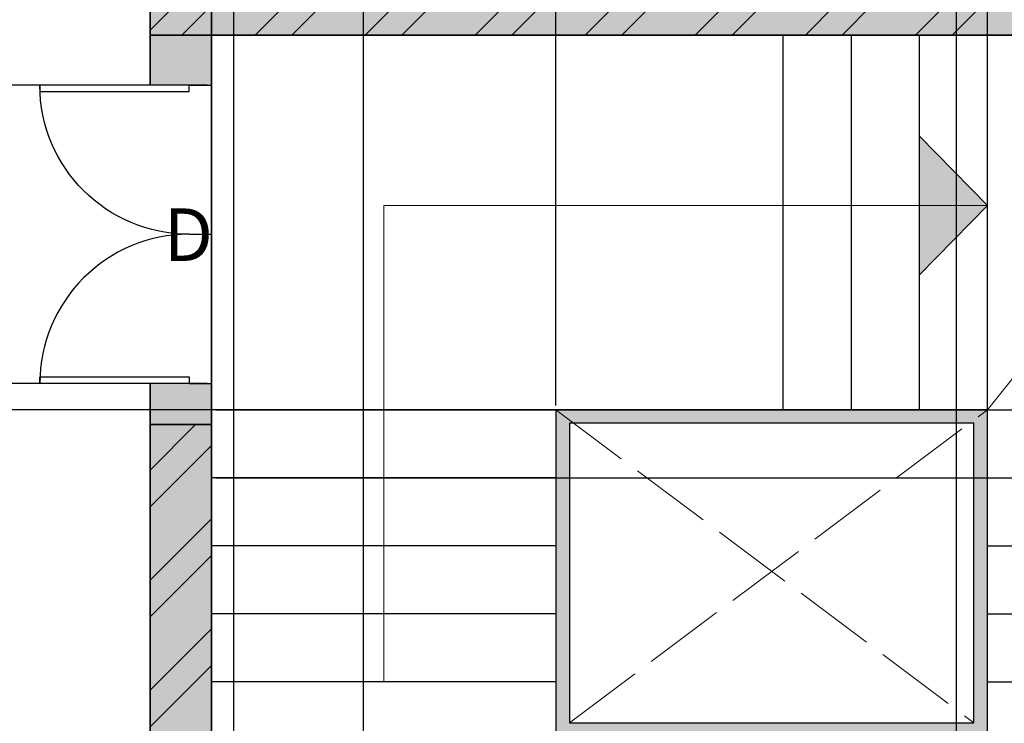
# Model space of a CAD drawing. Units: inches. Extents: x 1804 to 3296, y 909 to 2477.
# Tile 8 of 31: x 2130 to 2275, y 1226 to 1329. Entities that reach past the tile are written whole.
import ezdxf

# ---------------------------------------------------------------- set-up
doc = ezdxf.new("R2010")
doc.units = ezdxf.units.IN
doc.linetypes.add('ACAD_ISO02W100', pattern=[15, 12, -3])
for name, color, linetype, lineweight in [('A-ANNO-DIMS', 2, 'Continuous', 18), ('A-ANNO-SYMB', 7, 'Continuous', 18), ('A-ANNO-TTLB', 156, 'Continuous', 35), ('A-FLOR-PATT', 8, 'Continuous', 13), ('A-FLOR-STRS', 7, 'Continuous', 25), ('A-FLOR-STRS-OVHD', 8, 'ACAD_ISO02W100', 18), ('A-WALL-PATT', 10, 'Continuous', 13), ('DOOR', 30, 'Continuous', 25), ('TEXT', 190, 'Continuous', 18), ('WALL', 10, 'Continuous', 35)]:
    doc.layers.add(name, color=color, linetype=linetype, lineweight=lineweight)
doc.styles.get("Standard").update_dxf_attribs({"font": 'arial.ttf'})
doc.dimstyles.new('ISO-25', dxfattribs={"dimtxt": 5, "dimasz": 2.5, "dimexe": 1.25, "dimexo": 0.625, "dimtad": 1, "dimdec": 0, "dimlunit": 4, "dimtxsty": 'Standard', "dimcen": 2.5, "dimadec": 0, "dimazin": 0, "dimtfac": 1, "dimtdec": 0, "dimtmove": 0, "dimatfit": 3, "dimfxl": 1, "dimarcsym": 0})
pattern_1 = [(45, (0, 196.207), (-8.08223, 8.08223), []), (45, (5.388, 196.207), (-8.08223, 8.08223), [])]

# ---------------------------------------------------------------- blocks, each defined once
blk = doc.blocks.new('*U2')
for p, q in [((0, 0), (0, -6)), ((40, 0), (40, -6))]:
    blk.add_line(p, q)
blk.add_lwpolyline([(0, 0), (0, 40), (1.75, 40), (1.75, 0)], close=True)
blk.add_arc((0, 0), 40, 0, 90)
blk = doc.blocks.new('*D56')
at = {"layer": 'A-ANNO-DIMS', "color": 0, "lineweight": -2, "transparency": 16777216}
for p, q in [((2180.87, 1680.42), (2180.87, 975.89)), ((2268, 1680.42), (2268, 975.89)), ((2183.37, 977.14), (2265.5, 977.14))]:
    blk.add_line(p, q, dxfattribs=at)
at = {"layer": 'A-ANNO-DIMS', "color": 0, "lineweight": 100, "transparency": 16777216}
for points in [[(2183.37, 977.56), (2183.37, 976.72), (2180.87, 977.14)], [(2265.5, 977.56), (2265.5, 976.72), (2268, 977.14)]]:
    blk.add_solid(points, dxfattribs=at)
at = {"layer": 'Defpoints', "color": 0, "lineweight": 100, "transparency": 16777216}
for p in [(2180.87, 1681.04), (2268, 1681.04), (2268, 977.14)]:
    blk.add_point(p, dxfattribs=at)
at = {"layer": 'A-ANNO-DIMS', "color": 0, "transparency": 16777216, "insert": (2224.44, 980.32), "char_height": 5, "attachment_point": 5}
blk.add_mtext('7\'-3"', dxfattribs=at)
blk = doc.blocks.new('*D59')
at = {"layer": 'A-ANNO-DIMS', "color": 0, "lineweight": -2, "transparency": 16777216}
for p, q in [((2121.83, 1590.3), (2121.83, 975.89)), ((2161.83, 1590.3), (2161.83, 975.89)), ((2124.33, 977.14), (2159.33, 977.14))]:
    blk.add_line(p, q, dxfattribs=at)
at = {"layer": 'A-ANNO-DIMS', "color": 0, "lineweight": 100, "transparency": 16777216}
for points in [[(2124.33, 977.56), (2124.33, 976.72), (2121.83, 977.14)], [(2159.33, 977.56), (2159.33, 976.72), (2161.83, 977.14)]]:
    blk.add_solid(points, dxfattribs=at)
at = {"layer": 'Defpoints', "color": 0, "lineweight": 100, "transparency": 16777216}
for p in [(2121.83, 1590.92), (2161.83, 1590.92), (2161.83, 977.14)]:
    blk.add_point(p, dxfattribs=at)
at = {"layer": 'A-ANNO-DIMS', "color": 0, "transparency": 16777216, "insert": (2141.83, 980.32), "char_height": 5, "attachment_point": 5}
blk.add_mtext('3\'-4"', dxfattribs=at)
blk = doc.blocks.new('*D63')
at = {"layer": 'A-ANNO-DIMS', "color": 0, "lineweight": -2, "transparency": 16777216}
for p, q in [((2157.95, 1319.33), (1880.63, 1319.33)), ((1881.88, 1277.99), (1881.88, 1316.83)), ((2157.95, 1275.49), (1880.63, 1275.49))]:
    blk.add_line(p, q, dxfattribs=at)
at = {"layer": 'A-ANNO-DIMS', "color": 0, "lineweight": 100, "transparency": 16777216}
for points in [[(1881.47, 1316.83), (1882.3, 1316.83), (1881.88, 1319.33)], [(1881.47, 1277.99), (1882.3, 1277.99), (1881.88, 1275.49)]]:
    blk.add_solid(points, dxfattribs=at)
at = {"layer": 'Defpoints', "color": 0, "lineweight": 100, "transparency": 16777216}
for p in [(1881.88, 1319.33), (2158.58, 1319.33), (2158.58, 1275.49)]:
    blk.add_point(p, dxfattribs=at)
at = {"layer": 'A-ANNO-DIMS', "color": 0, "transparency": 16777216, "insert": (1878.7, 1297.41), "char_height": 5, "attachment_point": 5, "rotation": 90}
blk.add_mtext('3\'-8"', dxfattribs=at)
blk = doc.blocks.new('*D70')
at = {"layer": 'A-ANNO-DIMS', "color": 0, "lineweight": -2, "transparency": 16777216}
for p, q in [((2208.56, 1271.63), (1880.63, 1271.63)), ((1881.88, 1226.13), (1881.88, 1269.13)), ((2208.56, 1223.63), (1880.63, 1223.63))]:
    blk.add_line(p, q, dxfattribs=at)
at = {"layer": 'A-ANNO-DIMS', "color": 0, "lineweight": 100, "transparency": 16777216}
for points in [[(1881.47, 1269.13), (1882.3, 1269.13), (1881.88, 1271.63)], [(1881.47, 1226.13), (1882.3, 1226.13), (1881.88, 1223.63)]]:
    blk.add_solid(points, dxfattribs=at)
at = {"layer": 'Defpoints', "color": 0, "lineweight": 100, "transparency": 16777216}
for p in [(1881.88, 1271.63), (2209.19, 1271.63), (2209.19, 1223.63)]:
    blk.add_point(p, dxfattribs=at)
at = {"layer": 'A-ANNO-DIMS', "color": 0, "transparency": 16777216, "insert": (1878.7, 1247.63), "char_height": 5, "attachment_point": 5, "rotation": 90}
blk.add_mtext('4\'-0"', dxfattribs=at)
blk = doc.blocks.new('*D71')
at = {"layer": 'A-ANNO-DIMS', "color": 0, "lineweight": -2, "transparency": 16777216}
for p, q in [((2158.58, 1272.26), (2158.58, 1874.99)), ((2209.19, 1272.26), (2209.19, 1874.99)), ((2161.08, 1873.74), (2206.69, 1873.74))]:
    blk.add_line(p, q, dxfattribs=at)
at = {"layer": 'A-ANNO-DIMS', "color": 0, "lineweight": 100, "transparency": 16777216}
for points in [[(2161.08, 1874.15), (2161.08, 1873.32), (2158.58, 1873.74)], [(2206.69, 1874.15), (2206.69, 1873.32), (2209.19, 1873.74)]]:
    blk.add_solid(points, dxfattribs=at)
at = {"layer": 'Defpoints', "color": 0, "lineweight": 100, "transparency": 16777216}
for p in [(2209.19, 1873.74), (2158.58, 1271.63), (2209.19, 1271.63)]:
    blk.add_point(p, dxfattribs=at)
at = {"layer": 'A-ANNO-DIMS', "color": 0, "transparency": 16777216, "insert": (2183.88, 1876.95), "char_height": 5, "attachment_point": 5}
blk.add_mtext('4\'-2 1/2"', dxfattribs=at)
blk = doc.blocks.new('*D72')
at = {"layer": 'A-ANNO-DIMS', "color": 0, "lineweight": -2, "transparency": 16777216}
for p, q in [((2369.24, 1271.63), (2369.24, 1292.56)), ((2159.2, 1271.63), (2370.49, 1271.63)), ((2369.24, 1264.13), (2369.24, 1269.13)), ((2159.2, 1261.63), (2370.49, 1261.63))]:
    blk.add_line(p, q, dxfattribs=at)
at = {"layer": 'A-ANNO-DIMS', "color": 0, "lineweight": 100, "transparency": 16777216}
for points in [[(2368.82, 1269.13), (2369.65, 1269.13), (2369.24, 1271.63)], [(2368.82, 1264.13), (2369.65, 1264.13), (2369.24, 1261.63)]]:
    blk.add_solid(points, dxfattribs=at)
at = {"layer": 'Defpoints', "color": 0, "lineweight": 100, "transparency": 16777216}
for p in [(2158.58, 1271.63), (2369.24, 1271.63), (2158.58, 1261.63)]:
    blk.add_point(p, dxfattribs=at)
at = {"layer": 'A-ANNO-DIMS', "color": 0, "transparency": 16777216, "insert": (2366.06, 1283.35), "char_height": 5, "attachment_point": 5, "rotation": 90}
blk.add_mtext('0\'-10"', dxfattribs=at)
blk = doc.blocks.new('*D73')
at = {"layer": 'A-ANNO-DIMS', "color": 0, "lineweight": -2, "transparency": 16777216}
for p, q in [((2272.59, 1272.26), (2272.59, 1874.99)), ((2316.54, 1272.26), (2316.54, 1874.99)), ((2275.09, 1873.74), (2314.04, 1873.74))]:
    blk.add_line(p, q, dxfattribs=at)
at = {"layer": 'A-ANNO-DIMS', "color": 0, "lineweight": 100, "transparency": 16777216}
for points in [[(2275.09, 1874.15), (2275.09, 1873.32), (2272.59, 1873.74)], [(2314.04, 1874.15), (2314.04, 1873.32), (2316.54, 1873.74)]]:
    blk.add_solid(points, dxfattribs=at)
at = {"layer": 'Defpoints', "color": 0, "lineweight": 100, "transparency": 16777216}
for p in [(2316.54, 1873.74), (2272.59, 1271.63), (2316.54, 1271.63)]:
    blk.add_point(p, dxfattribs=at)
at = {"layer": 'A-ANNO-DIMS', "color": 0, "transparency": 16777216, "insert": (2294.56, 1876.92), "char_height": 5, "attachment_point": 5}
blk.add_mtext('3\'-8"', dxfattribs=at)
blk = doc.blocks.new('*D74')
at = {"layer": 'A-ANNO-DIMS', "color": 0, "lineweight": -2, "transparency": 16777216}
for p, q in [((2273.21, 1326.69), (2370.49, 1326.69)), ((2369.24, 1274.13), (2369.24, 1324.19)), ((2273.21, 1271.63), (2370.49, 1271.63))]:
    blk.add_line(p, q, dxfattribs=at)
at = {"layer": 'A-ANNO-DIMS', "color": 0, "lineweight": 100, "transparency": 16777216}
for points in [[(2368.82, 1324.19), (2369.65, 1324.19), (2369.24, 1326.69)], [(2368.82, 1274.13), (2369.65, 1274.13), (2369.24, 1271.63)]]:
    blk.add_solid(points, dxfattribs=at)
at = {"layer": 'Defpoints', "color": 0, "lineweight": 100, "transparency": 16777216}
for p in [(2272.59, 1326.69), (2369.24, 1326.69), (2272.59, 1271.63)]:
    blk.add_point(p, dxfattribs=at)
at = {"layer": 'A-ANNO-DIMS', "color": 0, "transparency": 16777216, "insert": (2366.11, 1299.16), "char_height": 5, "attachment_point": 5, "rotation": 90}
blk.add_mtext('4\'-7"', dxfattribs=at)

msp = doc.modelspace()

# ---------------------------------------------------------------- hatches: boundary and pattern name
at = {"layer": 'A-ANNO-SYMB'}
h = msp.add_hatch(color=256, dxfattribs=at)
h.dxf.hatch_style = 1
h.paths.add_polyline_path([(2262.59, 1311.85), (2262.59, 1301.66), (2272.59, 1301.66)])
h.paths.add_polyline_path([(2272.59, 1301.66), (2262.59, 1301.66), (2262.59, 1291.47)])
at = {"layer": 'A-ANNO-TTLB'}
h = msp.add_hatch(color=256, dxfattribs=at)
h.dxf.hatch_style = 1
h.paths.add_polyline_path([(3294.53, 2476.54), (1803.79, 2476.54), (1805.43, 909.47), (3296.17, 909.47)])
h.paths.add_polyline_path([(1811, 914.33), (1812.79, 2467.54), (3285.53, 2467.54), (3283.74, 914.33)], flags=16)
h.paths.add_polyline_path([(1925.58, 1062.77), (1925.58, 1138.07), (1925.58, 1539.88), (1925.58, 1793.38), (1925.58, 1830.04), (2325.54, 1830.04), (2325.54, 1793.38), (2325.54, 1586.42), (2325.54, 1138.07), (2325.54, 1062.77)], flags=0)
h.paths.add_polyline_path([(1997.22, 1029.4), (2008.85, 1037.96), (2008.85, 1020.84)], flags=0)
h.paths.add_polyline_path([(1934.58, 1138.07), (1934.58, 1147.07), (2078.77, 1147.07), (2078.77, 1138.07), (2060.94, 1138.07)], flags=0)
h.paths.add_polyline_path([(1944.35, 1138.07), (1944.35, 1147.07), (2056.05, 1147.07), (2056.05, 1138.07)], flags=0)
h.paths.add_polyline_path([(2222.24, 1037.96), (2233.87, 1029.4), (2222.24, 1020.84)], flags=0)
h.paths.add_polyline_path([(2061.94, 1139.07), (2061.94, 1146.07), (2077.77, 1146.07), (2077.77, 1139.07)], flags=0)
h.paths.add_polyline_path([(2149.58, 1138.07), (2149.58, 1269.44), (2158.58, 1269.44), (2158.58, 1326.69), (2149.58, 1326.69), (2149.58, 1340.94), (2139.6, 1340.94), (2139.6, 1434.25), (2149.58, 1434.25), (2149.58, 1447.36), (2158.58, 1447.36), (2158.58, 1423.87), (2158.58, 1408.06), (2198.46, 1408.06), (2198.46, 1412.56), (2282.65, 1412.56), (2282.65, 1465.94), (2316.54, 1465.94), (2316.54, 1590.92), (2192.86, 1590.92), (2192.86, 1595.3), (2291.17, 1595.3), (2291.17, 1590.92), (2316.54, 1590.92), (2316.54, 1784.38), (2300.24, 1784.38), (2300.24, 1757.47), (2268, 1757.47), (2268, 1681.04), (2180.87, 1681.04), (2180.87, 1757.47), (2148.63, 1757.47), (2148.63, 1784.38), (2119.08, 1784.38), (2119.08, 1585.58), (2114.58, 1585.58), (2114.58, 1784.38), (2064.11, 1784.38), (2046.28, 1784.38), (2046.28, 1760.38), (1958.58, 1760.38), (1958.58, 1664.38), (1934.58, 1664.38), (1934.58, 1784.38), (1934.58, 1793.38), (2046.28, 1793.38), (2064.11, 1793.38), (2119.08, 1793.38), (2230.78, 1793.38), (2230.78, 1784.38), (2268, 1784.38), (2300.24, 1784.38), (2316.54, 1784.38), (2316.54, 1590.92), (2316.54, 1373.73), (2316.54, 1138.07)], flags=0)
h.paths.add_polyline_path([(2209.19, 1166.63), (2209.19, 1175.63), (2158.58, 1175.63), (2209.19, 1223.63), (2209.19, 1231.63), (2183.88, 1231.63), (2183.88, 1301.66), (2242.59, 1301.66), (2242.59, 1326.69), (2316.54, 1326.69), (2272.59, 1271.63), (2272.59, 1223.63), (2316.54, 1175.63), (2272.59, 1175.63), (2272.59, 1166.63)], flags=0)
h.paths.add_polyline_path([(1947.77, 1345.22), (1947.77, 1457.48), (1991.2, 1457.48), (1991.2, 1451.7), (1991.2, 1352.18), (1991.2, 1345.22)], flags=0)
h.paths.add_polyline_path([(2209.19, 1271.63), (2262.59, 1271.63), (2262.59, 1311.85), (2272.59, 1301.66), (2272.59, 1271.63), (2269.92, 1269.63), (2270.59, 1269.63), (2270.59, 1225.63), (2211.19, 1225.63), (2211.19, 1269.63), (2211.86, 1269.63)], flags=0)
h.paths.add_polyline_path([(2000.34, 1378.21), (2000.34, 1429.71), (2025.22, 1429.71), (2025.22, 1378.21)], flags=0)
h.paths.add_polyline_path([(2001.34, 1379.21), (2001.34, 1428.71), (2024.22, 1428.71), (2024.22, 1379.21)], flags=0)
h.paths.add_polyline_path([(2012.34, 1390.21), (2012.34, 1417.71), (2013.22, 1417.71), (2013.22, 1390.21)], flags=0)
h.paths.add_polyline_path([(2237.56, 1331.19), (2237.56, 1340.18), (2238.62, 1340.18), (2238.62, 1386.84), (2241.04, 1386.84), (2242.06, 1386.84), (2242.06, 1408.06), (2316.54, 1331.19)], flags=0)
h.paths.add_polyline_path([(1953.73, 1464.35), (1953.73, 1498.59), (1981.74, 1498.59), (1981.74, 1464.35)], flags=0)
h.paths.add_polyline_path([(1987.63, 1462.08), (1987.63, 1500.95), (2104.07, 1500.95), (2104.07, 1462.08), (2099.27, 1462.08), (1993.6, 1462.08)], flags=0)
h.paths.add_polyline_path([(1956.06, 1481.47, -1), (1979.41, 1481.47, -1)], flags=0)
edge = h.paths.add_edge_path(flags=0)
edge.add_ellipse((2299.53, 1438.37), major_axis=(0.31, 21.36), ratio=0.670333, start_angle=0, end_angle=360)
h.paths.add_polyline_path([(2297.39, 1438.37, -1), (2301.67, 1438.37, -1)], flags=0)
h.paths.add_polyline_path([(2591.54, 1163.23), (2591.54, 1179.38), (2591.54, 1379.68), (2591.54, 1395.84), (2734.5, 1395.84), (2734.5, 1379.68), (2734.5, 1179.38), (2734.5, 1163.23)], flags=0)
h.paths.add_polyline_path([(2592.54, 1164.23), (2592.54, 1166.23), (2733.5, 1166.23), (2733.5, 1164.23)], flags=0)
h.paths.add_polyline_path([(2592.54, 1180.38), (2592.54, 1378.68), (2733.5, 1378.68), (2733.5, 1180.38)], flags=0)
h.paths.add_polyline_path([(2593.54, 1181.38), (2593.54, 1377.68), (2732.5, 1377.68), (2732.5, 1181.38)], flags=0)
h.paths.add_polyline_path([(2594.54, 1182.38), (2594.54, 1376.68), (2731.5, 1376.68), (2731.5, 1182.38)], flags=0)
h.paths.add_polyline_path([(1936.95, 1697.46), (1936.95, 1736.46), (1955.41, 1736.46), (1955.41, 1697.46)], flags=0)
h.paths.add_polyline_path([(1938.48, 1718.36), (1938.48, 1734.92), (1953.65, 1734.92), (1953.65, 1718.36)], flags=0)
h.paths.add_polyline_path([(1944.75, 1726.64, -1), (1947.37, 1726.64, -1)], flags=0)
h.paths.add_polyline_path([(2592.54, 1394.84), (2733.5, 1394.84), (2733.5, 1392.84), (2592.54, 1392.84)], flags=0)
h.paths.add_polyline_path([(1976.61, 1762.5), (1976.61, 1781.44), (2012.79, 1781.44), (2012.79, 1762.5)], flags=0)
h.paths.add_polyline_path([(1979.57, 1771.97, -1), (1991.39, 1771.97, -1)], flags=0)
h.paths.add_polyline_path([(1995.36, 1771.97, -1), (2007.18, 1771.97, -1)], flags=0)
h.paths.add_polyline_path([(2251.51, 1744.53), (2268, 1730.05), (2251.51, 1730.05)], flags=0)
h.paths.add_polyline_path([(2047.28, 1785.38), (2047.28, 1792.38), (2063.11, 1792.38), (2063.11, 1785.38)], flags=0)
h.paths.add_polyline_path([(2155.08, 1770.92, -1), (2174.42, 1770.92, -1)], flags=0)
h.paths.add_polyline_path([(2188.59, 1758.27), (2188.59, 1772.81), (2222.3, 1772.81), (2222.3, 1758.27)], flags=0)
h.paths.add_polyline_path([(2223.97, 1758.27), (2223.97, 1772.81), (2257.68, 1772.81), (2257.68, 1758.27)], flags=0)
h.paths.add_polyline_path([(2274.45, 1770.92, -1), (2293.8, 1770.92, -1)], flags=0)
h.paths.add_polyline_path([(2591.54, 1582.09), (2591.54, 1782.39), (2734.5, 1782.39), (2734.5, 1582.09)], flags=0)
h.paths.add_polyline_path([(2592.54, 1583.09), (2592.54, 1781.39), (2733.5, 1781.39), (2733.5, 1583.09)], flags=0)
h.paths.add_polyline_path([(2593.54, 1584.09), (2593.54, 1780.39), (2732.5, 1780.39), (2732.5, 1584.09)], flags=0)
h.paths.add_polyline_path([(2594.54, 1585.09), (2594.54, 1779.39), (2731.5, 1779.39), (2731.5, 1585.09)], flags=0)
h.paths.add_polyline_path([(1922.17, 1978.79), (1922.17, 2295.08), (1922.17, 2296.08), (2115.67, 2296.08), (2115.67, 2384.31), (2115.67, 2385.31), (2322.12, 2385.31), (2323.12, 2385.31), (2323.12, 1979.79), (2323.12, 1978.79), (1923.17, 1978.79)], flags=0)
h.paths.add_polyline_path([(1922.17, 1978.79), (1922.17, 2051.31), (1922.17, 2214.86), (1922.17, 2296.08), (2115.67, 2296.08), (2115.67, 2385.31), (2323.12, 2385.31), (2323.12, 2280.42), (2323.12, 1978.79), (2115.67, 1978.79)], flags=0)
h.paths.add_polyline_path([(1923.17, 1979.79), (1923.17, 2050.31), (2115.67, 2050.31), (2115.67, 2051.31), (1923.17, 2051.31), (1923.17, 2213.86), (1923.17, 2214.86), (1923.17, 2295.08), (1990.02, 2295.08), (1990.02, 2214.86), (1991.02, 2214.86), (1991.02, 2295.08), (2115.67, 2295.08), (2115.67, 1979.79), (2116.67, 1979.79), (2116.67, 2304.18), (2116.67, 2384.31), (2322.12, 2384.31), (2322.12, 2280.42), (2322.12, 1979.79), (2115.67, 1979.79)], flags=0)
h.paths.add_polyline_path([(2972.46, 1192.5), (2972.46, 1196.92), (2995.47, 1196.92), (2995.47, 1255.47), (2995.09, 1255.47), (2987.42, 1249.39), (2980.08, 1255.47), (2978.05, 1255.47), (2978.05, 1257.24), (2995.47, 1257.24), (2995.47, 1261.58), (3015.37, 1261.58), (3015.37, 1333.28), (3015.37, 1414.4), (3032.82, 1414.4), (3032.82, 1333.28), (3032.82, 1261.58), (3052.66, 1261.58), (3052.66, 1255.47), (3079.86, 1255.47), (3078.72, 1254.57), (3081.47, 1252.29), (3078.56, 1249.99), (3075.81, 1252.26), (3072.57, 1249.69), (3070.36, 1251.52), (3067.67, 1249.39), (3060.34, 1255.47), (3052.66, 1255.47), (3052.66, 1196.92), (3054.58, 1196.92), (3074, 1196.92), (3074, 1192.5), (3052.66, 1192.5), (2995.47, 1192.5)], flags=0)
h.paths.add_polyline_path([(2490.75, 1979.27), (2490.75, 1980.27), (2596.87, 1980.27), (2596.87, 2051.8), (2596.87, 2052.8), (2596.87, 2216.35), (2596.87, 2297.57), (2717.32, 2297.57), (2710.57, 2305.62), (2724.07, 2305.62), (2717.32, 2297.57), (2782.37, 2297.57), (2782.37, 2395.8), (3006.82, 2395.8), (3006.82, 1981.27), (3093.73, 1981.27), (3093.73, 1980.27), (3047.51, 1980.27), (3046.37, 1979.37), (3049.11, 1977.1), (3046.2, 1974.79), (3043.46, 1977.07), (3040.21, 1974.49), (3038, 1976.32), (3035.32, 1974.2), (3027.98, 1980.27), (2871.83, 1980.27), (2871.83, 1981.27), (2791.37, 1981.27), (2791.37, 2050.8), (2597.87, 2050.8), (2597.87, 1980.27), (2597.87, 1979.27), (2546.27, 1979.27), (2545.12, 1978.37), (2547.87, 1976.1), (2544.96, 1973.79), (2542.22, 1976.07), (2538.97, 1973.49), (2536.76, 1975.32), (2534.07, 1973.2), (2526.74, 1979.27)], flags=0)
h.paths.add_polyline_path([(2597.87, 2051.8), (2606.87, 2051.8), (2606.87, 2258.39), (2597.87, 2258.39), (2597.87, 2296.57), (2606.87, 2296.57), (2606.87, 2262.39), (2782.37, 2262.39), (2782.37, 2296.57), (2790.37, 2296.57), (2790.37, 2262.39), (2791.37, 2262.39), (2791.37, 2305.67), (2791.37, 2385.8), (2996.82, 2385.8), (2996.82, 2339.85), (3006.82, 2339.85), (3006.82, 2250.12), (2997.82, 2250.12), (2997.82, 1981.27), (2996.82, 1981.27), (2872.83, 1981.27), (2872.83, 1991.8), (2871.83, 1991.8), (2871.83, 2050.8), (2790.37, 2050.8), (2597.87, 2050.8)], flags=0)
h.paths.add_polyline_path([(2179.93, 2153.92), (2179.93, 2353.97), (2259.98, 2353.97), (2259.98, 2153.92)], flags=0)
h.paths.add_polyline_path([(2180.93, 2154.92), (2180.93, 2352.97), (2258.98, 2352.97), (2258.98, 2154.92)], flags=0)
h.paths.add_polyline_path([(2960.87, 1608.49), (2960.87, 1753.62), (3070.9, 1753.62), (3070.9, 1608.49)], flags=0)
h.paths.add_polyline_path([(2961.87, 1609.49), (2961.87, 1752.62), (3069.9, 1752.62), (3069.9, 1609.49)], flags=0)
h.paths.add_polyline_path([(2962.87, 1610.49), (2962.87, 1751.62), (3068.9, 1751.62), (3068.9, 1610.49)], flags=0)
h.paths.add_polyline_path([(2963.87, 1611.49), (2963.87, 1750.62), (3067.9, 1750.62), (3067.9, 1611.49)], flags=0)
h.paths.add_polyline_path([(2782.37, 2051.8), (2782.37, 2216.32), (2791.37, 2216.32), (2791.37, 2051.8), (2872.83, 2051.8), (2872.83, 2068.56), (2884.67, 2068.56), (2884.67, 2085.33), (2896.51, 2085.33), (2896.51, 2102.09), (2908.36, 2102.09), (2908.36, 2118.85), (2920.2, 2118.85), (2920.2, 2135.62), (2932.05, 2135.62), (2932.05, 2145.3), (2925.08, 2145.3), (2925.08, 2203.2), (2996.82, 2203.2), (2996.82, 2145.3), (2953.82, 2145.3), (2872.83, 2051.8), (2790.37, 2051.8)], flags=0)
h.paths.add_polyline_path([(2717.32, 2238.65), (2710.57, 2246.7), (2724.07, 2246.7)], flags=0)
h.paths.add_polyline_path([(2003.09, 1122.79), (2017.16, 1122.79), (2017.16, 1138.74), (2003.09, 1138.74)], flags=8)
h.paths.add_polyline_path([(2174.76, 1792.72), (2188.83, 1792.72), (2188.83, 1808.66), (2174.76, 1808.66)], flags=8)
h.paths.add_polyline_path([(1987.95, 1792.51), (2002.02, 1792.51), (2002.02, 1808.45), (1987.95, 1808.45)], flags=8)
h.paths.add_polyline_path([(2148.79, 1289.26), (2160.46, 1289.26), (2160.46, 1305.2), (2148.79, 1305.2)], flags=8)
h.paths.add_polyline_path([(2115.36, 1133.57), (2127.04, 1133.57), (2127.04, 1149.51), (2115.36, 1149.51)], flags=8)
h.paths.add_polyline_path([(2237.58, 1421.48), (2249.25, 1421.48), (2249.25, 1437.43), (2237.58, 1437.43)], flags=8)
h.paths.add_polyline_path([(2134.99, 1584.32), (2146.66, 1584.32), (2146.66, 1600.26), (2134.99, 1600.26)], flags=8)
h.paths.add_polyline_path([(2101.95, 1557.31), (2113.62, 1557.31), (2113.62, 1573.25), (2101.95, 1573.25)], flags=8)
h.paths.add_polyline_path([(2937.85, 1156.77), (3120.41, 1156.77), (3120.41, 1185.72), (2937.85, 1185.72)], flags=8)
h.paths.add_polyline_path([(2980.71, 1786.71), (3050.06, 1786.71), (3050.06, 1802.66), (2980.71, 1802.66)], flags=8)
h.paths.add_polyline_path([(2869.28, 1661.96), (2938.62, 1661.96), (2938.62, 1690.8), (2869.28, 1690.8)], flags=8)
h.paths.add_polyline_path([(3092.27, 1674.86), (3161.62, 1674.86), (3161.62, 1690.8), (3092.27, 1690.8)], flags=8)
h.paths.add_polyline_path([(2980.71, 1674.86), (3050.06, 1674.86), (3050.06, 1690.8), (2980.71, 1690.8)], flags=8)
h.paths.add_polyline_path([(2649.07, 1678.23), (2674.53, 1678.23), (2674.53, 1714.76), (2649.07, 1714.76)], flags=8)
h.paths.add_polyline_path([(2530.84, 1981.63), (2549.13, 1981.63), (2549.13, 1997.57), (2530.84, 1997.57)], flags=8)
h.paths.add_polyline_path([(3031.29, 1981.77), (3049.58, 1981.77), (3049.58, 1997.71), (3031.29, 1997.71)], flags=8)
h.paths.add_polyline_path([(2715.38, 1911.9), (2851.54, 1911.9), (2851.54, 1940.85), (2715.38, 1940.85)], flags=8)
h.paths.add_polyline_path([(2015.23, 1927.36), (2205.42, 1927.36), (2205.42, 1956.3), (2015.23, 1956.3)], flags=8)
h.paths.add_polyline_path([(2671.84, 2057.84), (2702.75, 2057.84), (2702.75, 2073.79), (2671.84, 2073.79)], flags=8)
h.paths.add_polyline_path([(2678.5, 2316.52), (2765.26, 2316.52), (2765.26, 2332.46), (2678.5, 2332.46)], flags=8)
h.paths.add_polyline_path([(2678.48, 2271.96), (2736.41, 2271.96), (2736.41, 2287.9), (2678.48, 2287.9)], flags=8)
h.paths.add_polyline_path([(2019.2, 972.79), (2243.21, 972.79), (2243.21, 1001.74), (2019.2, 1001.74)], flags=8)
h.paths.add_polyline_path([(2097.06, 1021.56), (2132.16, 1021.56), (2132.16, 1037.51), (2097.06, 1037.51)], flags=8)
h.paths.add_polyline_path([(2182.47, 1360.48), (2207.35, 1360.48), (2207.35, 1376.42), (2182.47, 1376.42)], flags=8)
h.paths.add_polyline_path([(2261.12, 1361.77), (2295.01, 1361.77), (2295.01, 1377.71), (2261.12, 1377.71)], flags=8)
h.paths.add_polyline_path([(2245.75, 1511.51), (2278.44, 1511.51), (2278.44, 1527.46), (2245.75, 1527.46)], flags=8)
h.paths.add_polyline_path([(1991.16, 1296.29), (2060.51, 1296.29), (2060.51, 1312.23), (1991.16, 1312.23)], flags=8)
h.paths.add_polyline_path([(2187, 1651.35), (2246.71, 1651.35), (2246.71, 1667.29), (2187, 1667.29)], flags=8)
h.paths.add_polyline_path([(1976.49, 1684.81), (2068.63, 1684.81), (2068.63, 1700.76), (1976.49, 1700.76)], flags=8)
at = {"layer": 'A-FLOR-PATT'}
h = msp.add_hatch(color=256, dxfattribs=at)
h.dxf.hatch_style = 1
h.paths.add_polyline_path([(2272.59, 1271.63), (2209.19, 1271.63), (2211.86, 1269.63), (2269.92, 1269.63)], flags=17)
h.paths.add_polyline_path([(2211.19, 1269.63), (2211.86, 1269.63), (2209.19, 1271.63), (2209.19, 1223.63), (2272.59, 1223.63), (2272.59, 1271.63), (2269.92, 1269.63), (2270.59, 1269.63), (2270.59, 1225.63), (2211.19, 1225.63)])
at = {"layer": 'A-WALL-PATT'}
h = msp.add_hatch(color=256, dxfattribs=at)
h.dxf.hatch_style = 1
h.paths.add_polyline_path([(2119.08, 1544.38), (1925.58, 1544.38), (1925.58, 1539.88), (2119.08, 1539.88)])
h.paths.add_polyline_path([(2119.08, 1545.58), (2114.58, 1545.58), (2114.58, 1544.38), (2119.08, 1544.38)])
h.paths.add_polyline_path([(1965.87, 1658.79), (1965.87, 1679.09), (1955.57, 1679.09), (1955.57, 1658.79)], flags=9)
h.paths.add_polyline_path([(2293.18, 1677.29), (2293.18, 1697.58), (2282.88, 1697.58), (2282.88, 1677.29)], flags=9)
h.paths.add_polyline_path([(2271.13, 1545.23), (2287.53, 1545.23), (2287.53, 1555.53), (2271.13, 1555.53)], flags=9)
h.paths.add_polyline_path([(2303.26, 1488.52), (2303.26, 1508.82), (2292.95, 1508.82), (2292.95, 1488.52)], flags=9)
h.paths.add_polyline_path([(2271.13, 1393.15), (2287.53, 1393.15), (2287.53, 1403.45), (2271.13, 1403.45)], flags=9)
h.paths.add_polyline_path([(2306.48, 1361.45), (2306.48, 1377.86), (2296.18, 1377.86), (2296.18, 1361.45)], flags=9)
h.paths.add_polyline_path([(2174.54, 1361.45), (2174.54, 1377.86), (2164.23, 1377.86), (2164.23, 1361.45)], flags=9)
h.paths.add_polyline_path([(1968.21, 1333.34), (1968.21, 1353.64), (1957.91, 1353.64), (1957.91, 1333.34)], flags=9)
h.paths.add_polyline_path([(2003.09, 1122.79), (2017.16, 1122.79), (2017.16, 1138.74), (2003.09, 1138.74)], flags=9)
h.paths.add_polyline_path([(2174.76, 1792.72), (2188.83, 1792.72), (2188.83, 1808.66), (2174.76, 1808.66)], flags=9)
h.paths.add_polyline_path([(1987.95, 1792.51), (2002.02, 1792.51), (2002.02, 1808.45), (1987.95, 1808.45)], flags=9)
h.paths.add_polyline_path([(2148.79, 1289.26), (2160.46, 1289.26), (2160.46, 1305.2), (2148.79, 1305.2)], flags=9)
h.paths.add_polyline_path([(2115.36, 1133.57), (2127.04, 1133.57), (2127.04, 1149.51), (2115.36, 1149.51)], flags=9)
h.paths.add_polyline_path([(2237.58, 1421.48), (2249.25, 1421.48), (2249.25, 1437.43), (2237.58, 1437.43)], flags=9)
h.paths.add_polyline_path([(2134.99, 1584.32), (2146.66, 1584.32), (2146.66, 1600.26), (2134.99, 1600.26)], flags=9)
h.paths.add_polyline_path([(2101.95, 1557.31), (2113.62, 1557.31), (2113.62, 1573.25), (2101.95, 1573.25)], flags=9)
h.paths.add_polyline_path([(2937.85, 1156.77), (3120.41, 1156.77), (3120.41, 1185.72), (2937.85, 1185.72)], flags=9)
h.paths.add_polyline_path([(2980.71, 1786.71), (3050.06, 1786.71), (3050.06, 1802.66), (2980.71, 1802.66)], flags=9)
h.paths.add_polyline_path([(2869.28, 1661.96), (2938.62, 1661.96), (2938.62, 1690.8), (2869.28, 1690.8)], flags=9)
h.paths.add_polyline_path([(3092.27, 1674.86), (3161.62, 1674.86), (3161.62, 1690.8), (3092.27, 1690.8)], flags=9)
h.paths.add_polyline_path([(2980.71, 1674.86), (3050.06, 1674.86), (3050.06, 1690.8), (2980.71, 1690.8)], flags=9)
h.paths.add_polyline_path([(2649.07, 1678.23), (2674.53, 1678.23), (2674.53, 1714.76), (2649.07, 1714.76)], flags=9)
h.paths.add_polyline_path([(2530.84, 1981.63), (2549.13, 1981.63), (2549.13, 1997.57), (2530.84, 1997.57)], flags=9)
h.paths.add_polyline_path([(3031.29, 1981.77), (3049.58, 1981.77), (3049.58, 1997.71), (3031.29, 1997.71)], flags=9)
h.paths.add_polyline_path([(2715.38, 1911.9), (2851.54, 1911.9), (2851.54, 1940.85), (2715.38, 1940.85)], flags=9)
h.paths.add_polyline_path([(2015.23, 1927.36), (2205.42, 1927.36), (2205.42, 1956.3), (2015.23, 1956.3)], flags=9)
h.paths.add_polyline_path([(2671.84, 2057.84), (2702.75, 2057.84), (2702.75, 2073.79), (2671.84, 2073.79)], flags=9)
h.paths.add_polyline_path([(2678.5, 2316.52), (2765.26, 2316.52), (2765.26, 2332.46), (2678.5, 2332.46)], flags=9)
h.paths.add_polyline_path([(2678.48, 2271.96), (2736.41, 2271.96), (2736.41, 2287.9), (2678.48, 2287.9)], flags=9)
h.paths.add_polyline_path([(2019.2, 972.79), (2243.21, 972.79), (2243.21, 1001.74), (2019.2, 1001.74)], flags=9)
h.paths.add_polyline_path([(2097.06, 1021.56), (2132.16, 1021.56), (2132.16, 1037.51), (2097.06, 1037.51)], flags=9)
h.paths.add_polyline_path([(2182.47, 1360.48), (2207.35, 1360.48), (2207.35, 1376.42), (2182.47, 1376.42)], flags=9)
h.paths.add_polyline_path([(2261.12, 1361.77), (2295.01, 1361.77), (2295.01, 1377.71), (2261.12, 1377.71)], flags=9)
h.paths.add_polyline_path([(2245.75, 1511.51), (2278.44, 1511.51), (2278.44, 1527.46), (2245.75, 1527.46)], flags=9)
h.paths.add_polyline_path([(1991.16, 1296.29), (2060.51, 1296.29), (2060.51, 1312.23), (1991.16, 1312.23)], flags=9)
h.paths.add_polyline_path([(2187, 1651.35), (2246.71, 1651.35), (2246.71, 1667.29), (2187, 1667.29)], flags=9)
h.paths.add_polyline_path([(1976.49, 1684.81), (2068.63, 1684.81), (2068.63, 1700.76), (1976.49, 1700.76)], flags=9)
h = msp.add_hatch(color=256, dxfattribs=at)
h.dxf.hatch_style = 1
h.paths.add_polyline_path([(2149.58, 1147.07), (2141.21, 1147.07), (2141.21, 1144.07), (2141.21, 1138.07), (2149.58, 1138.07)])
h.paths.add_polyline_path([(2101.21, 1144.07, -0.01877), (2101.32, 1147.07), (2078.77, 1147.07), (2078.77, 1138.07), (2101.21, 1138.07)])
h.paths.add_polyline_path([(2060.94, 1147.07), (2056.05, 1147.07), (2056.05, 1138.07), (2060.94, 1138.07)])
h.paths.add_polyline_path([(1944.35, 1147.07), (1934.58, 1147.07), (1934.58, 1138.07), (1944.35, 1138.07)])
h.paths.add_polyline_path([(2158.58, 1269.44), (2149.58, 1269.44), (2149.58, 1138.07), (2158.58, 1138.07)])
h.paths.add_polyline_path([(2003.09, 1122.79), (2017.16, 1122.79), (2017.16, 1138.74), (2003.09, 1138.74)], flags=9)
h.paths.add_polyline_path([(2174.76, 1792.72), (2188.83, 1792.72), (2188.83, 1808.66), (2174.76, 1808.66)], flags=9)
h.paths.add_polyline_path([(1987.95, 1792.51), (2002.02, 1792.51), (2002.02, 1808.45), (1987.95, 1808.45)], flags=9)
h.paths.add_polyline_path([(2148.79, 1289.26), (2160.46, 1289.26), (2160.46, 1305.2), (2148.79, 1305.2)], flags=9)
h.paths.add_polyline_path([(2115.36, 1133.57), (2127.04, 1133.57), (2127.04, 1149.51), (2115.36, 1149.51)], flags=9)
h.paths.add_polyline_path([(2237.58, 1421.48), (2249.25, 1421.48), (2249.25, 1437.43), (2237.58, 1437.43)], flags=9)
h.paths.add_polyline_path([(2134.99, 1584.32), (2146.66, 1584.32), (2146.66, 1600.26), (2134.99, 1600.26)], flags=9)
h.paths.add_polyline_path([(2101.95, 1557.31), (2113.62, 1557.31), (2113.62, 1573.25), (2101.95, 1573.25)], flags=9)
h.paths.add_polyline_path([(2937.85, 1156.77), (3120.41, 1156.77), (3120.41, 1185.72), (2937.85, 1185.72)], flags=9)
h.paths.add_polyline_path([(2980.71, 1786.71), (3050.06, 1786.71), (3050.06, 1802.66), (2980.71, 1802.66)], flags=9)
h.paths.add_polyline_path([(2869.28, 1661.96), (2938.62, 1661.96), (2938.62, 1690.8), (2869.28, 1690.8)], flags=9)
h.paths.add_polyline_path([(3092.27, 1674.86), (3161.62, 1674.86), (3161.62, 1690.8), (3092.27, 1690.8)], flags=9)
h.paths.add_polyline_path([(2980.71, 1674.86), (3050.06, 1674.86), (3050.06, 1690.8), (2980.71, 1690.8)], flags=9)
h.paths.add_polyline_path([(2649.07, 1678.23), (2674.53, 1678.23), (2674.53, 1714.76), (2649.07, 1714.76)], flags=9)
h.paths.add_polyline_path([(2530.84, 1981.63), (2549.13, 1981.63), (2549.13, 1997.57), (2530.84, 1997.57)], flags=9)
h.paths.add_polyline_path([(3031.29, 1981.77), (3049.58, 1981.77), (3049.58, 1997.71), (3031.29, 1997.71)], flags=9)
h.paths.add_polyline_path([(2715.38, 1911.9), (2851.54, 1911.9), (2851.54, 1940.85), (2715.38, 1940.85)], flags=9)
h.paths.add_polyline_path([(2015.23, 1927.36), (2205.42, 1927.36), (2205.42, 1956.3), (2015.23, 1956.3)], flags=9)
h.paths.add_polyline_path([(2671.84, 2057.84), (2702.75, 2057.84), (2702.75, 2073.79), (2671.84, 2073.79)], flags=9)
h.paths.add_polyline_path([(2678.5, 2316.52), (2765.26, 2316.52), (2765.26, 2332.46), (2678.5, 2332.46)], flags=9)
h.paths.add_polyline_path([(2678.48, 2271.96), (2736.41, 2271.96), (2736.41, 2287.9), (2678.48, 2287.9)], flags=9)
h.paths.add_polyline_path([(2019.2, 972.79), (2243.21, 972.79), (2243.21, 1001.74), (2019.2, 1001.74)], flags=9)
h.paths.add_polyline_path([(2097.06, 1021.56), (2132.16, 1021.56), (2132.16, 1037.51), (2097.06, 1037.51)], flags=9)
h.paths.add_polyline_path([(2182.47, 1360.48), (2207.35, 1360.48), (2207.35, 1376.42), (2182.47, 1376.42)], flags=9)
h.paths.add_polyline_path([(2261.12, 1361.77), (2295.01, 1361.77), (2295.01, 1377.71), (2261.12, 1377.71)], flags=9)
h.paths.add_polyline_path([(2245.75, 1511.51), (2278.44, 1511.51), (2278.44, 1527.46), (2245.75, 1527.46)], flags=9)
h.paths.add_polyline_path([(1991.16, 1296.29), (2060.51, 1296.29), (2060.51, 1312.23), (1991.16, 1312.23)], flags=9)
h.paths.add_polyline_path([(2187, 1651.35), (2246.71, 1651.35), (2246.71, 1667.29), (2187, 1667.29)], flags=9)
h.paths.add_polyline_path([(1976.49, 1684.81), (2068.63, 1684.81), (2068.63, 1700.76), (1976.49, 1700.76)], flags=9)
h = msp.add_hatch(color=256, dxfattribs=at)
h.dxf.hatch_style = 1
h.paths.add_polyline_path([(2158.58, 1275.49), (2155.29, 1275.49), (2149.58, 1275.49), (2149.58, 1269.44), (2158.58, 1269.44)])
h.paths.add_polyline_path([(2158.58, 1326.69), (2149.58, 1326.69), (2149.58, 1319.33), (2155.29, 1319.33), (2158.58, 1319.33)])
h.paths.add_polyline_path([(2158.58, 1402.2), (2158.58, 1423.87), (2158.58, 1447.36), (2149.58, 1447.36), (2149.58, 1423.87), (2149.58, 1340.94), (2149.58, 1326.69), (2158.58, 1326.69), (2158.58, 1354.23)])
h.paths.add_polyline_path([(1965.87, 1658.79), (1965.87, 1679.09), (1955.57, 1679.09), (1955.57, 1658.79)], flags=9)
h.paths.add_polyline_path([(2293.18, 1677.29), (2293.18, 1697.58), (2282.88, 1697.58), (2282.88, 1677.29)], flags=9)
h.paths.add_polyline_path([(2271.13, 1545.23), (2287.53, 1545.23), (2287.53, 1555.53), (2271.13, 1555.53)], flags=9)
h.paths.add_polyline_path([(2303.26, 1488.52), (2303.26, 1508.82), (2292.95, 1508.82), (2292.95, 1488.52)], flags=9)
h.paths.add_polyline_path([(2271.13, 1393.15), (2287.53, 1393.15), (2287.53, 1403.45), (2271.13, 1403.45)], flags=9)
h.paths.add_polyline_path([(2306.48, 1361.45), (2306.48, 1377.86), (2296.18, 1377.86), (2296.18, 1361.45)], flags=9)
h.paths.add_polyline_path([(2189.9, 1340.62), (2206.31, 1340.62), (2206.31, 1350.92), (2189.9, 1350.92)], flags=9)
h.paths.add_polyline_path([(2174.54, 1361.45), (2174.54, 1377.86), (2164.23, 1377.86), (2164.23, 1361.45)], flags=9)
h.paths.add_polyline_path([(2304.24, 1240.8), (2304.24, 1261.09), (2293.94, 1261.09), (2293.94, 1240.8)], flags=9)
h.paths.add_polyline_path([(2227.19, 1188.73), (2247.49, 1188.73), (2247.49, 1199.03), (2227.19, 1199.03)], flags=9)
h.paths.add_polyline_path([(2181.93, 1144.21), (2181.93, 1160.62), (2171.63, 1160.62), (2171.63, 1144.21)], flags=9)
h.paths.add_polyline_path([(1968.21, 1333.34), (1968.21, 1353.64), (1957.91, 1353.64), (1957.91, 1333.34)], flags=9)
h.paths.add_polyline_path([(2029.78, 1203.53), (2053.95, 1203.53), (2053.95, 1213.83), (2029.78, 1213.83)], flags=9)
h.paths.add_polyline_path([(2576.51, 1671.88), (2576.51, 1692.17), (2566.21, 1692.17), (2566.21, 1671.88)], flags=9)
h.paths.add_polyline_path([(2566.99, 1269.67), (2566.99, 1289.96), (2556.68, 1289.96), (2556.68, 1269.67)], flags=9)
h.paths.add_polyline_path([(2581.85, 1269.17), (2581.85, 1289.46), (2571.54, 1289.46), (2571.54, 1269.17)], flags=9)
h.paths.add_polyline_path([(2650.71, 1409.75), (2674.89, 1409.75), (2674.89, 1420.05), (2650.71, 1420.05)], flags=9)
h.paths.add_polyline_path([(2003.09, 1122.79), (2017.16, 1122.79), (2017.16, 1138.74), (2003.09, 1138.74)], flags=9)
h.paths.add_polyline_path([(2174.76, 1792.72), (2188.83, 1792.72), (2188.83, 1808.66), (2174.76, 1808.66)], flags=9)
h.paths.add_polyline_path([(1987.95, 1792.51), (2002.02, 1792.51), (2002.02, 1808.45), (1987.95, 1808.45)], flags=9)
h.paths.add_polyline_path([(2148.79, 1289.26), (2160.46, 1289.26), (2160.46, 1305.2), (2148.79, 1305.2)], flags=9)
h.paths.add_polyline_path([(2115.36, 1133.57), (2127.04, 1133.57), (2127.04, 1149.51), (2115.36, 1149.51)], flags=9)
h.paths.add_polyline_path([(2237.58, 1421.48), (2249.25, 1421.48), (2249.25, 1437.43), (2237.58, 1437.43)], flags=9)
h.paths.add_polyline_path([(2134.99, 1584.32), (2146.66, 1584.32), (2146.66, 1600.26), (2134.99, 1600.26)], flags=9)
h.paths.add_polyline_path([(2101.95, 1557.31), (2113.62, 1557.31), (2113.62, 1573.25), (2101.95, 1573.25)], flags=9)
h.paths.add_polyline_path([(2937.85, 1156.77), (3120.41, 1156.77), (3120.41, 1185.72), (2937.85, 1185.72)], flags=9)
h.paths.add_polyline_path([(2980.71, 1786.71), (3050.06, 1786.71), (3050.06, 1802.66), (2980.71, 1802.66)], flags=9)
h.paths.add_polyline_path([(2869.28, 1661.96), (2938.62, 1661.96), (2938.62, 1690.8), (2869.28, 1690.8)], flags=9)
h.paths.add_polyline_path([(3092.27, 1674.86), (3161.62, 1674.86), (3161.62, 1690.8), (3092.27, 1690.8)], flags=9)
h.paths.add_polyline_path([(2980.71, 1674.86), (3050.06, 1674.86), (3050.06, 1690.8), (2980.71, 1690.8)], flags=9)
h.paths.add_polyline_path([(2649.07, 1678.23), (2674.53, 1678.23), (2674.53, 1714.76), (2649.07, 1714.76)], flags=9)
h.paths.add_polyline_path([(2530.84, 1981.63), (2549.13, 1981.63), (2549.13, 1997.57), (2530.84, 1997.57)], flags=9)
h.paths.add_polyline_path([(3031.29, 1981.77), (3049.58, 1981.77), (3049.58, 1997.71), (3031.29, 1997.71)], flags=9)
h.paths.add_polyline_path([(2715.38, 1911.9), (2851.54, 1911.9), (2851.54, 1940.85), (2715.38, 1940.85)], flags=9)
h.paths.add_polyline_path([(2015.23, 1927.36), (2205.42, 1927.36), (2205.42, 1956.3), (2015.23, 1956.3)], flags=9)
h.paths.add_polyline_path([(2671.84, 2057.84), (2702.75, 2057.84), (2702.75, 2073.79), (2671.84, 2073.79)], flags=9)
h.paths.add_polyline_path([(2678.5, 2316.52), (2765.26, 2316.52), (2765.26, 2332.46), (2678.5, 2332.46)], flags=9)
h.paths.add_polyline_path([(2678.48, 2271.96), (2736.41, 2271.96), (2736.41, 2287.9), (2678.48, 2287.9)], flags=9)
h.paths.add_polyline_path([(2019.2, 972.79), (2243.21, 972.79), (2243.21, 1001.74), (2019.2, 1001.74)], flags=9)
h.paths.add_polyline_path([(2097.06, 1021.56), (2132.16, 1021.56), (2132.16, 1037.51), (2097.06, 1037.51)], flags=9)
h.paths.add_polyline_path([(2182.47, 1360.48), (2207.35, 1360.48), (2207.35, 1376.42), (2182.47, 1376.42)], flags=9)
h.paths.add_polyline_path([(2261.12, 1361.77), (2295.01, 1361.77), (2295.01, 1377.71), (2261.12, 1377.71)], flags=9)
h.paths.add_polyline_path([(2245.75, 1511.51), (2278.44, 1511.51), (2278.44, 1527.46), (2245.75, 1527.46)], flags=9)
h.paths.add_polyline_path([(1991.16, 1296.29), (2060.51, 1296.29), (2060.51, 1312.23), (1991.16, 1312.23)], flags=9)
h.paths.add_polyline_path([(2187, 1651.35), (2246.71, 1651.35), (2246.71, 1667.29), (2187, 1667.29)], flags=9)
h.paths.add_polyline_path([(1976.49, 1684.81), (2068.63, 1684.81), (2068.63, 1700.76), (1976.49, 1700.76)], flags=9)
h = msp.add_hatch(dxfattribs=at)
h.set_pattern_fill('ANSI32', color=256, scale=1.2)
h.set_pattern_definition(pattern_1)
h.paths.add_polyline_path([(1934.58, 1784.38), (1934.58, 1793.38), (1925.58, 1793.38), (1925.58, 1539.88), (2119.08, 1539.88), (2119.08, 1545.58), (2114.58, 1545.58), (2114.58, 1544.38), (1934.58, 1544.38)])
h.paths.add_polyline_path([(2114.58, 1793.38), (2064.11, 1793.38), (2064.11, 1784.38), (2114.58, 1784.38)], flags=17)
h.paths.add_polyline_path([(2325.54, 1793.38), (2230.78, 1793.38), (2230.78, 1784.38), (2268, 1784.38), (2300.24, 1784.38), (2316.54, 1784.38), (2316.54, 1590.92), (2316.54, 1586.42), (2325.54, 1586.42)])
h.paths.add_polyline_path([(1944.35, 1147.07), (1934.58, 1147.07), (1934.58, 1138.07), (1944.35, 1138.07)])
h.paths.add_polyline_path([(2101.21, 1144.07, -0.01877), (2101.32, 1147.07), (2078.77, 1147.07), (2078.77, 1138.07), (2101.21, 1138.07)])
h.paths.add_polyline_path([(1934.58, 1539.88), (1925.58, 1539.88), (1925.58, 1138.07), (1934.58, 1138.07), (1934.58, 1147.07)])
h.paths.add_polyline_path([(2325.54, 1586.42), (2316.54, 1586.42), (2316.54, 1373.73), (2316.54, 1138.07), (2325.54, 1138.07), (2325.54, 1228.97)])
h.paths.add_polyline_path([(2158.58, 1423.87), (2158.58, 1447.36), (2149.58, 1447.36), (2149.58, 1423.87), (2149.58, 1340.94), (2149.58, 1326.69), (2158.58, 1326.69), (2158.58, 1354.23), (2158.58, 1402.2)])
h.paths.add_polyline_path([(2316.54, 1412.56), (2282.65, 1412.56), (2273.09, 1412.56), (2273.09, 1408.06), (2316.54, 1408.06)])
h.paths.add_polyline_path([(2273.09, 1412.56), (2242.06, 1412.56), (2242.06, 1408.06), (2273.09, 1408.06)])
h.paths.add_polyline_path([(2237.56, 1412.56), (2198.46, 1412.56), (2198.46, 1408.06), (2237.56, 1408.06)])
h.paths.add_polyline_path([(2242.06, 1408.06), (2237.56, 1408.06), (2237.56, 1386.84), (2242.06, 1386.84)])
h.paths.add_polyline_path([(2242.06, 1412.56), (2237.56, 1412.56), (2237.56, 1408.06), (2242.06, 1408.06)])
h.paths.add_polyline_path([(2158.58, 1269.44), (2149.58, 1269.44), (2149.58, 1138.07), (2158.58, 1138.07)])
h.paths.add_polyline_path([(2149.58, 1147.07), (2141.21, 1147.07), (2141.21, 1144.07), (2141.21, 1138.07), (2149.58, 1138.07)])
h.paths.add_polyline_path([(2272.59, 1175.63), (2209.19, 1175.63), (2209.19, 1166.63), (2272.59, 1166.63)])
h.paths.add_polyline_path([(2237.56, 1446.21), (2242.06, 1446.21), (2242.06, 1586.42), (2237.56, 1586.42)])
h.paths.add_polyline_path([(2242.06, 1414.58), (2237.56, 1414.58), (2237.56, 1412.56), (2242.06, 1412.56)])
h = msp.add_hatch(color=256, dxfattribs=at)
h.dxf.hatch_style = 1
h.paths.add_polyline_path([(2114.58, 1793.38), (2064.11, 1793.38), (2064.11, 1784.38), (2114.58, 1784.38)])
h.paths.add_polyline_path([(2119.08, 1793.38), (2114.58, 1793.38), (2114.58, 1585.58), (2119.08, 1585.58)])
h.paths.add_polyline_path([(2325.54, 1793.38), (2230.78, 1793.38), (2230.78, 1784.38), (2268, 1784.38), (2316.54, 1784.38), (2316.54, 1590.92), (2316.54, 1586.42), (2325.54, 1586.42)])
h.paths.add_polyline_path([(2316.54, 1331.19), (2158.58, 1331.19), (2158.58, 1326.69), (2316.54, 1326.69)])
h.paths.add_polyline_path([(2242.06, 1408.06), (2237.56, 1408.06), (2237.56, 1386.84), (2242.06, 1386.84)])
h.paths.add_polyline_path([(2242.06, 1412.56), (2237.56, 1412.56), (2237.56, 1408.06), (2242.06, 1408.06)])
h.paths.add_polyline_path([(2237.56, 1412.56), (2198.46, 1412.56), (2198.46, 1408.06), (2237.56, 1408.06)])
h.paths.add_polyline_path([(2273.09, 1412.56), (2242.06, 1412.56), (2242.06, 1408.06), (2273.09, 1408.06)])
h.paths.add_polyline_path([(2316.54, 1412.56), (2282.65, 1412.56), (2273.09, 1412.56), (2273.09, 1408.06), (2316.54, 1408.06)])
h.paths.add_polyline_path([(2325.54, 1586.42), (2316.54, 1586.42), (2316.54, 1373.73), (2316.54, 1138.07), (2325.54, 1138.07), (2325.54, 1228.97)])
h.paths.add_polyline_path([(2272.59, 1175.63), (2209.19, 1175.63), (2209.19, 1166.63), (2272.59, 1166.63)])
h = msp.add_hatch(dxfattribs=at)
h.set_pattern_fill('ANSI32', color=256, scale=1.2)
h.set_pattern_definition(pattern_1)
h.paths.add_polyline_path([(2316.54, 1331.19), (2158.58, 1331.19), (2158.58, 1326.69), (2316.54, 1326.69)])
h.paths.add_polyline_path([(2242.06, 1340.18), (2237.56, 1340.18), (2237.56, 1331.19), (2242.06, 1331.19)])
h.paths.add_polyline_path([(2242.06, 1408.06), (2237.56, 1408.06), (2237.56, 1386.84), (2242.06, 1386.84)])

# ---------------------------------------------------------------- linework, layer by layer
at = {"layer": 'A-ANNO-SYMB'}
for p, q in [((2272.59, 1301.66), (2262.59, 1311.85)), ((2183.88, 1231.63), (2183.88, 1301.66)), ((2183.88, 1301.66), (2272.59, 1301.66)), ((2272.59, 1301.66), (2262.59, 1291.47))]:
    msp.add_line(p, q, dxfattribs=at)
at = {"layer": 'A-FLOR-STRS'}
for p, q in [((2242.59, 1271.63), (2242.59, 1326.69)), ((2252.59, 1271.63), (2252.59, 1326.69)), ((2262.59, 1271.63), (2262.59, 1326.69)), ((2272.59, 1271.63), (2272.59, 1326.69)), ((2209.19, 1271.63), (2158.58, 1271.63)), ((2272.59, 1271.63), (2209.19, 1271.63)), ((2209.19, 1271.63), (2209.19, 1223.63)), ((2272.59, 1223.63), (2272.59, 1271.63)), ((2272.59, 1271.63), (2316.54, 1271.63)), ((2270.59, 1269.63), (2211.19, 1269.63)), ((2211.19, 1269.63), (2211.19, 1225.63)), ((2270.59, 1225.63), (2270.59, 1269.63)), ((2209.19, 1261.63), (2158.58, 1261.63)), ((2272.59, 1261.63), (2316.54, 1261.63)), ((2209.19, 1251.63), (2158.58, 1251.63)), ((2272.59, 1251.63), (2316.54, 1251.63)), ((2209.19, 1241.63), (2158.58, 1241.63)), ((2209.19, 1241.63), (2158.58, 1241.63)), ((2272.59, 1241.63), (2316.54, 1241.63)), ((2209.19, 1231.63), (2158.58, 1231.63)), ((2272.59, 1231.63), (2316.54, 1231.63)), ((2211.19, 1225.63), (2270.59, 1225.63))]:
    msp.add_line(p, q, dxfattribs=at)
at = {"layer": 'A-FLOR-STRS-OVHD'}
for p, q in [((2272.59, 1271.63), (2316.54, 1326.69)), ((2209.19, 1271.63), (2270.59, 1225.63)), ((2211.19, 1225.63), (2272.59, 1271.63))]:
    msp.add_line(p, q, dxfattribs=at)
at = {"layer": 'WALL'}
for p, q in [((2149.58, 1326.69), (2149.58, 1355.19)), ((2158.58, 1138.07), (2158.58, 1354.23)), ((2158.58, 1326.69), (2149.58, 1326.69)), ((2149.58, 1326.69), (2149.58, 1319.33)), ((2158.58, 1326.69), (2316.54, 1326.69)), ((2149.58, 1269.44), (2149.58, 1275.49)), ((2149.58, 1138.07), (2149.58, 1269.44)), ((2149.58, 1269.44), (2158.58, 1269.44))]:
    msp.add_line(p, q, dxfattribs=at)

# ---------------------------------------------------------------- block references
at = {"layer": 'DOOR', "yscale": 0.5479986435874215, "zscale": 0.5479986435874215, "rotation": 90}
for p, xscale in [((2155.29, 1319.33), -0.5479986435874215), ((2155.29, 1275.49), 0.5479986435874215)]:
    msp.add_blockref('*U2', p, dxfattribs=dict(at, xscale=xscale))

# ---------------------------------------------------------------- texts
at = {"layer": 'TEXT', "insert": (2151.55, 1301.22), "char_height": 7.74, "attachment_point": 1}
msp.add_mtext_dynamic_manual_height_columns('D', width=163.3261, gutter_width=38.69, heights=[0], dxfattribs=at)

# ---------------------------------------------------------------- dimensions: what is measured, and where the dimension line sits
at = {"layer": 'A-ANNO-DIMS'}
for base, p1, p2, picture, middle in [((2209.19, 1873.74), (2158.58, 1271.63), (2209.19, 1271.63), '*D71', (2183.88, 1876.95)), ((2316.5375, 1873.7362), (2272.5886, 1271.6342), (2316.5375, 1271.6342), '*D73', (2294.563, 1876.9158)), ((2268, 977.14), (2180.87, 1681.04), (2268, 1681.04), '*D56', (2224.44, 980.32)), ((2161.83, 977.14), (2121.83, 1590.92), (2161.83, 1590.92), '*D59', (2141.83, 980.32))]:
    dim = msp.add_linear_dim(base=base, p1=p1, p2=p2, dimstyle='ISO-25', override={"dimdec": 1, "dimlfac": 1, "dimrnd": 0, "dimzin": 1, "dimdsep": 46, "dimlunit": 4, "dimfrac": 2}, dxfattribs=at)
    dim.commit()
    dim.dimension.update_dxf_attribs({"geometry": picture, "text_midpoint": middle})
for base, p1, p2, picture, middle in [((2369.24, 1326.69), (2272.59, 1271.63), (2272.59, 1326.69), '*D74', (2366.11, 1299.16)), ((1881.88, 1319.33), (2158.58, 1275.49), (2158.58, 1319.33), '*D63', (1878.7, 1297.41)), ((2369.24, 1271.63), (2158.58, 1261.63), (2158.58, 1271.63), '*D72', (2366.06, 1283.35)), ((1881.88, 1271.63), (2209.19, 1223.63), (2209.19, 1271.63), '*D70', (1878.7, 1247.63))]:
    dim = msp.add_linear_dim(base=base, p1=p1, p2=p2, angle=90, dimstyle='ISO-25', override={"dimdec": 1, "dimlfac": 1, "dimrnd": 0, "dimzin": 1, "dimdsep": 46, "dimlunit": 4, "dimfrac": 2}, dxfattribs=at)
    dim.commit()
    dim.dimension.update_dxf_attribs({"geometry": picture, "text_midpoint": middle})

doc.saveas('drawing.dxf')
